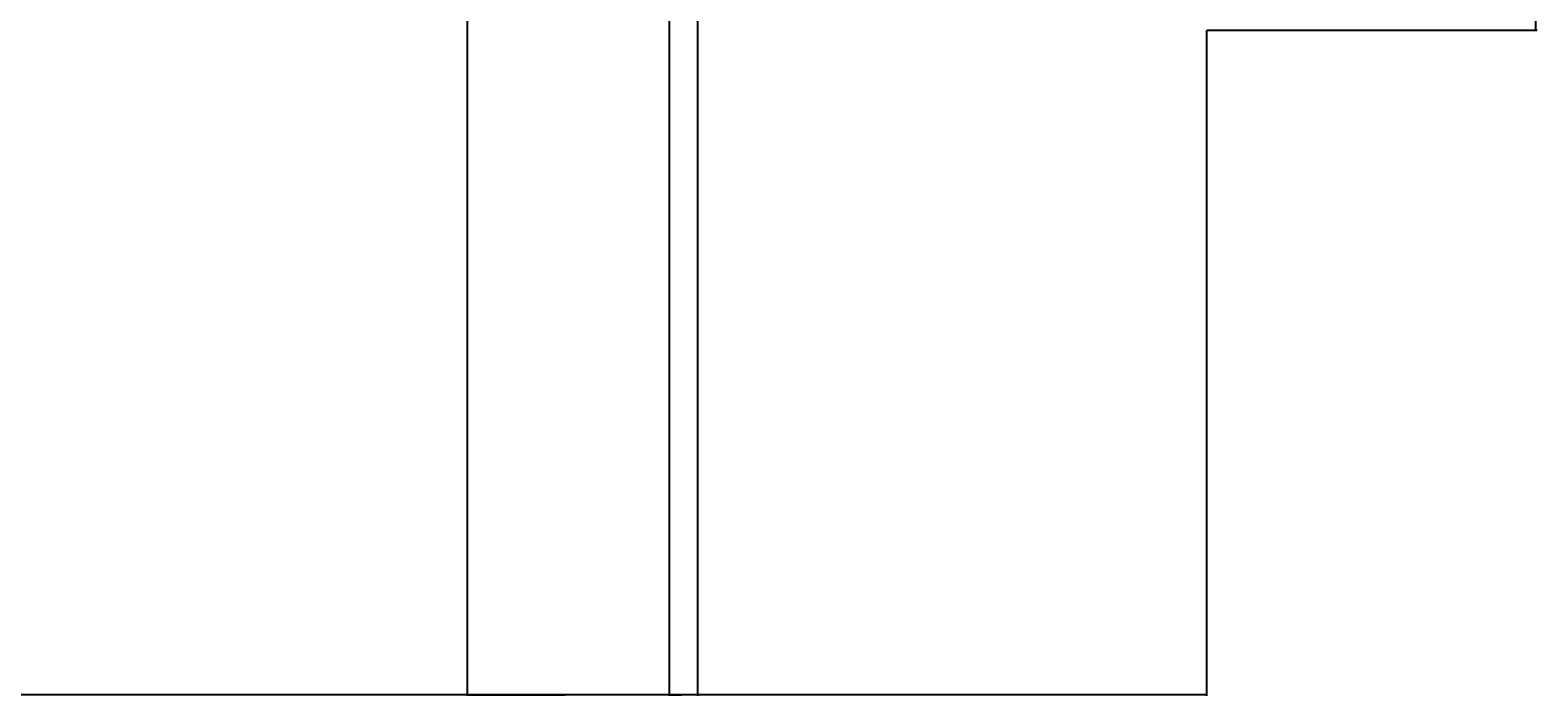
# Model space of a CAD drawing. Units: inches. Extents: x 5375 to 6084, y 16106 to 17259.
# Tile 9 of 32: x 5844 to 6084, y 16106 to 16212. Entities that reach past the tile are written whole.
import ezdxf

# ---------------------------------------------------------------- set-up
doc = ezdxf.new("R2010")
doc.units = ezdxf.units.IN
doc.layers.add('A-ANNO-DIMS', color=2, linetype='Continuous', lineweight=18)
doc.styles.get("Standard").update_dxf_attribs({"font": 'arial.ttf'})
doc.dimstyles.get("Standard").update_dxf_attribs({"dimtxt": 0.18, "dimasz": 0.18, "dimexe": 0.18, "dimexo": 0.0625, "dimgap": 0.09, "dimtad": 0, "dimtih": 1, "dimtoh": 1, "dimdec": 4, "dimzin": 0, "dimdsep": 46, "dimtxsty": 'Standard', "dimcen": 0.09, "dimadec": 0, "dimazin": 0, "dimtfac": 1, "dimtdec": 4, "dimtofl": 0, "dimtmove": 0, "dimatfit": 3, "dimfxl": 1, "dimtolj": 1, "dimtzin": 0, "dimarcsym": 0})

# ---------------------------------------------------------------- blocks, each defined once
blk = doc.blocks.new('*D30')
at = {"layer": 'A-ANNO-DIMS', "color": 0, "lineweight": -2, "transparency": 16777216}
for p, q in [((5470.62, 16212.32), (5470.62, 16106.48)), ((6031.62, 16212.32), (6031.62, 16106.48)), ((5470.8, 16106.66), (5750.85, 16106.66)), ((6031.44, 16106.66), (5751.39, 16106.66))]:
    blk.add_line(p, q, dxfattribs=at)
at = {"layer": 'A-ANNO-DIMS', "color": 0, "transparency": 16777216}
for points in [[(5470.8, 16106.69), (5470.8, 16106.63), (5470.62, 16106.66)], [(6031.44, 16106.69), (6031.44, 16106.63), (6031.62, 16106.66)]]:
    blk.add_solid(points, dxfattribs=at)
at = {"layer": 'Defpoints', "color": 0, "transparency": 16777216}
for p in [(5470.62, 16212.38), (6031.62, 16212.38), (6031.62, 16106.66)]:
    blk.add_point(p, dxfattribs=at)
at = {"layer": 'A-ANNO-DIMS', "color": 0, "transparency": 16777216, "insert": (5751.12, 16106.66), "char_height": 0.18, "attachment_point": 5}
blk.add_mtext('\\A1;561', dxfattribs=at)
blk = doc.blocks.new('*D31')
at = {"layer": 'A-ANNO-DIMS', "color": 0, "lineweight": -2, "transparency": 16777216}
for p, q in [((6031.68, 17206.58), (6084.2, 17206.58)), ((6084.02, 17206.4), (6084.02, 16709.66)), ((6084.02, 16212.56), (6084.02, 16709.3)), ((6031.68, 16212.38), (6084.2, 16212.38))]:
    blk.add_line(p, q, dxfattribs=at)
at = {"layer": 'A-ANNO-DIMS', "color": 0, "transparency": 16777216}
for points in [[(6083.99, 17206.4), (6084.05, 17206.4), (6084.02, 17206.58)], [(6083.99, 16212.56), (6084.05, 16212.56), (6084.02, 16212.38)]]:
    blk.add_solid(points, dxfattribs=at)
at = {"layer": 'Defpoints', "color": 0, "transparency": 16777216}
for p in [(6031.62, 17206.58), (6084.02, 17206.58), (6031.62, 16212.38)]:
    blk.add_point(p, dxfattribs=at)
at = {"layer": 'A-ANNO-DIMS', "color": 0, "transparency": 16777216, "insert": (6084.02, 16709.48), "char_height": 0.18, "attachment_point": 5}
blk.add_mtext('\\A1;994.2', dxfattribs=at)
blk = doc.blocks.new('*D44')
at = {"layer": 'A-ANNO-DIMS', "color": 0, "lineweight": -2, "transparency": 16777216}
for p, q in [((5914, 16886.53), (5914, 16106.48)), ((5946.12, 16886.53), (5946.12, 16106.48)), ((5914.18, 16106.66), (5929.6, 16106.66)), ((5945.94, 16106.66), (5930.53, 16106.66))]:
    blk.add_line(p, q, dxfattribs=at)
at = {"layer": 'A-ANNO-DIMS', "color": 0, "transparency": 16777216}
for points in [[(5914.18, 16106.69), (5914.18, 16106.63), (5914, 16106.66)], [(5945.94, 16106.69), (5945.94, 16106.63), (5946.12, 16106.66)]]:
    blk.add_solid(points, dxfattribs=at)
at = {"layer": 'Defpoints', "color": 0, "transparency": 16777216}
for p in [(5914, 16886.6), (5946.12, 16886.6), (5914, 16106.66)]:
    blk.add_point(p, dxfattribs=at)
at = {"layer": 'A-ANNO-DIMS', "color": 0, "transparency": 16777216, "insert": (5930.06, 16106.66), "char_height": 0.18, "attachment_point": 5}
blk.add_mtext('\\A1;32.117', dxfattribs=at)
blk = doc.blocks.new('*D46')
at = {"layer": 'A-ANNO-DIMS', "color": 0, "lineweight": -2, "transparency": 16777216}
for p, q in [((5946.12, 16771.52), (5946.12, 16106.48)), ((5950.62, 16771.52), (5950.62, 16106.48)), ((5946.3, 16106.66), (5948.11, 16106.66)), ((5950.44, 16106.66), (5948.63, 16106.66))]:
    blk.add_line(p, q, dxfattribs=at)
at = {"layer": 'A-ANNO-DIMS', "color": 0, "transparency": 16777216}
for points in [[(5946.3, 16106.69), (5946.3, 16106.63), (5946.12, 16106.66)], [(5950.44, 16106.69), (5950.44, 16106.63), (5950.62, 16106.66)]]:
    blk.add_solid(points, dxfattribs=at)
at = {"layer": 'Defpoints', "color": 0, "transparency": 16777216}
for p in [(5946.12, 16771.58), (5950.62, 16771.58), (5950.62, 16106.66)]:
    blk.add_point(p, dxfattribs=at)
at = {"layer": 'A-ANNO-DIMS', "color": 0, "transparency": 16777216, "insert": (5948.37, 16106.66), "char_height": 0.18, "attachment_point": 5}
blk.add_mtext('\\A1;4.5', dxfattribs=at)

msp = doc.modelspace()

# ---------------------------------------------------------------- dimensions: what is measured, and where the dimension line sits
at = {"layer": 'A-ANNO-DIMS'}
dim = msp.add_linear_dim(base=(6084.0199, 17206.5793), p1=(6031.6199, 16212.3785), p2=(6031.6199, 17206.5793), angle=90, dimstyle='Standard', override={"dimdec": 1, "dimlfac": 1, "dimrnd": 0, "dimzin": 0, "dimdsep": 46, "dimlunit": 2}, dxfattribs=at)
dim.commit()
dim.dimension.update_dxf_attribs({"geometry": '*D31', "text_midpoint": (6084.0199, 16709.4789)})
for base, p1, p2, override, picture, middle in [((5914.0033, 16106.6631), (5946.1199, 16886.5956), (5914.0033, 16886.5956), {"dimdec": 3, "dimlfac": 1, "dimrnd": 0, "dimzin": 0, "dimdsep": 46, "dimlunit": 2}, '*D44', (5930.0616, 16106.6631)), ((5950.6199, 16106.6631), (5946.1199, 16771.5793), (5950.6199, 16771.5793), {"dimdec": 1, "dimlfac": 1, "dimrnd": 0, "dimzin": 0, "dimdsep": 46, "dimlunit": 2}, '*D46', (5948.3699, 16106.6631)), ((6031.6199, 16106.6631), (5470.6199, 16212.3785), (6031.6199, 16212.3785), {"dimdec": 0, "dimlfac": 1, "dimrnd": 0, "dimzin": 0, "dimdsep": 46, "dimlunit": 2}, '*D30', (5751.1199, 16106.6631))]:
    dim = msp.add_linear_dim(base=base, p1=p1, p2=p2, dimstyle='Standard', override=override, dxfattribs=at)
    dim.commit()
    dim.dimension.update_dxf_attribs({"geometry": picture, "text_midpoint": middle})

doc.saveas('drawing.dxf')
